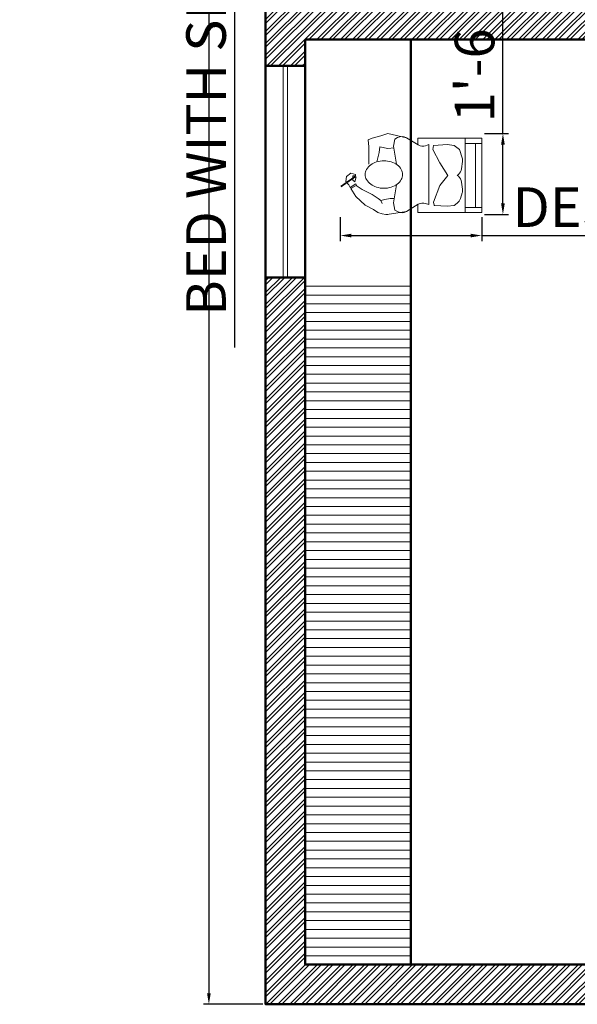
# Model space of a CAD drawing. Units: inches. Extents: x 3590 to 5167, y 65 to 1917.
# Tile 16 of 100: x 3590 to 3716, y 1326 to 1549. Entities that reach past the tile are written whole.
import ezdxf

# ---------------------------------------------------------------- set-up
doc = ezdxf.new("R2010")
doc.units = ezdxf.units.IN
for name, color, linetype, lineweight in [('A-ANNO-DIMS', 2, 'Continuous', 18), ('A-FURN', 21, 'Continuous', 18), ('A-GLAZ', 4, 'Continuous', 18), ('A-WALL', 7, 'Continuous', 50), ('A-WALL-PATT', 251, 'Continuous', 13)]:
    doc.layers.add(name, color=color, linetype=linetype, lineweight=lineweight)
doc.styles.get("Standard").update_dxf_attribs({"font": 'arial.ttf'})
doc.dimstyles.new('ISO-25', dxfattribs={"dimtxt": 9, "dimasz": 2.5, "dimexe": 1.25, "dimexo": 0.625, "dimtad": 1, "dimdec": 1, "dimlunit": 3, "dimtxsty": 'Standard', "dimcen": 2.5, "dimadec": 0, "dimazin": 0, "dimtfac": 1, "dimtdec": 1, "dimtmove": 0, "dimatfit": 3, "dimfxl": 1, "dimarcsym": 0})

# ---------------------------------------------------------------- blocks, each defined once
blk = doc.blocks.new('*D6')
at = {"layer": 'A-ANNO-DIMS', "color": 0, "lineweight": -2, "transparency": 16777216}
for p, q in [((3644.89, 1806), (3631.39, 1806)), ((3632.64, 1803.5), (3632.64, 1328.5)), ((3644.89, 1326), (3631.39, 1326))]:
    blk.add_line(p, q, dxfattribs=at)
at = {"layer": 'A-ANNO-DIMS', "color": 0, "transparency": 16777216}
for points in [[(3632.22, 1803.5), (3633.06, 1803.5), (3632.64, 1806)], [(3632.22, 1328.5), (3633.06, 1328.5), (3632.64, 1326)]]:
    blk.add_solid(points, dxfattribs=at)
at = {"layer": 'Defpoints', "color": 0, "transparency": 16777216}
for p in [(3645.51, 1806), (3632.64, 1326), (3645.51, 1326)]:
    blk.add_point(p, dxfattribs=at)
at = {"layer": 'A-ANNO-DIMS', "color": 0, "transparency": 16777216, "insert": (3627.42, 1566), "char_height": 9, "attachment_point": 5, "rotation": 90}
blk.add_mtext("40'", dxfattribs=at)
blk = doc.blocks.new('DESK-CHAIR')
for p, q in [((3674.9, 1522.4), (3674.54, 1520.79)), ((3675.51, 1522.74), (3674.9, 1522.4)), ((3680.2, 1521.08), (3677.49, 1522.71)), ((3694.59, 1522.58), (3680.09, 1522.58)), ((3680.09, 1522.58), (3680.09, 1521.15)), ((3694.59, 1505.74), (3694.59, 1522.58)), ((3674.54, 1520.79), (3675.25, 1516.67)), ((3682.6, 1521.15), (3681.85, 1520.9)), ((3682.6, 1521.15), (3682.6, 1507.53)), ((3682.6, 1507.53), (3682.6, 1521.15)), ((3683.49, 1520.07), (3683.66, 1520.91)), ((3685.1, 1517.02), (3683.49, 1520.07)), ((3683.73, 1520.97), (3686.72, 1521.15)), ((3686.72, 1521.15), (3688.33, 1520.97)), ((3688.33, 1520.97), (3689.58, 1520.07)), ((3689.58, 1520.07), (3690.17, 1518.15)), ((3686.89, 1514.16), (3685.1, 1517.02)), ((3690.24, 1517.32), (3690.04, 1515.67)), ((3685.1, 1511.83), (3686.89, 1514.16)), ((3689.31, 1514.37), (3689.04, 1514.16)), ((3689.31, 1513.95), (3689.04, 1514.16)), ((3664.74, 1511.43), (3666.04, 1512.26)), ((3665.07, 1511.29), (3664.74, 1511.43)), ((3664.84, 1511.19), (3666.07, 1511.86)), ((3666.04, 1509.36), (3664.84, 1511.19)), ((3666.04, 1512.26), (3666.24, 1511.79)), ((3666.07, 1511.86), (3667.43, 1510.93)), ((3667.43, 1510.93), (3669.7, 1509.83)), ((3674.54, 1507.89), (3675.25, 1512.01)), ((3683.67, 1508.07), (3685.1, 1511.83)), ((3690.24, 1511), (3690.04, 1512.64)), ((3668.13, 1507.37), (3666.04, 1509.36)), ((3669.7, 1509.83), (3671.06, 1508.9)), ((3671.06, 1508.9), (3671.66, 1508.47)), ((3689.78, 1508.89), (3690.17, 1510.17)), ((3670.06, 1506.4), (3668.13, 1507.37)), ((3671.66, 1508.47), (3671.96, 1507.77)), ((3674.9, 1506.27), (3674.54, 1507.89)), ((3680.2, 1507.6), (3677.49, 1505.97)), ((3680.09, 1507.53), (3680.09, 1505.74)), ((3682.6, 1507.53), (3681.85, 1507.78)), ((3683.8, 1507.4), (3683.67, 1508.07)), ((3683.88, 1507.34), (3686.72, 1507.17)), ((3686.72, 1507.17), (3688.33, 1507.35)), ((3688.33, 1507.35), (3689.03, 1507.86)), ((3677.49, 1505.97), (3673.14, 1505.31)), ((3675.51, 1505.94), (3674.9, 1506.27)), ((3680.09, 1505.74), (3694.59, 1505.74))]:
    blk.add_line(p, q)
for points in [[(3677.49, 1522.71), (3673.28, 1523.65), (3671.67, 1523.12), (3669.7, 1522.58), (3668.81, 1522.22), (3668.99, 1520.61), (3668.99, 1519), (3668.99, 1516.67)], [(3664.74, 1511.43), (3664.42, 1512.05), (3663.77, 1512.78), (3663.87, 1513.9), (3664.88, 1514.67), (3665.92, 1514.37), (3665.9, 1514.02), (3665.32, 1514.02), (3665.3, 1513.1), (3665.82, 1512.66), (3666.07, 1513.84)], [(3671.66, 1508.47), (3672.6, 1508.69), (3673.82, 1508.93), (3674.7, 1508.93)], [(3670.06, 1506.4), (3671.04, 1505.75), (3672.02, 1505.46), (3672.8, 1505.31), (3673.24, 1505.31)]]:
    blk.add_lwpolyline(points)
at = {"const_width": 0.39}
blk.add_lwpolyline([(3666.01, 1513.98), (3662.61, 1511.61)], dxfattribs=at)
for centre, radius, start, end in [((3676.47, 1521), 1.98, 59.0235, 119.0669), ((3681.22, 1522.78), 1.98, 239.0235, 288.4436), ((3683.74, 1520.89), 0.0779, 93.3682, 168.6956), ((3683.74, 1520.89), 0.0779, 93.3682, 168.6956), ((3688.27, 1517.56), 1.98, 352.8785, 17.0946), ((3688.07, 1515.92), 1.98, 308.6739, 352.8785), ((3688.07, 1512.4), 1.98, 7.1215, 51.3261), ((3688.27, 1510.75), 1.98, 342.9054, 7.1215), ((3687.88, 1509.47), 1.98, 305.5514, 342.9054), ((3681.22, 1505.89), 1.98, 71.5564, 120.9765), ((3683.88, 1507.42), 0.0779, 191.3044, 266.6318), ((3676.47, 1507.67), 1.98, 240.9331, 300.9765)]:
    blk.add_arc(centre, radius, start, end)
blk = doc.blocks.new('*D286')
at = {"layer": 'A-ANNO-DIMS', "color": 0, "lineweight": -2, "transparency": 16777216}
for p, q in [((3653.89, 1797), (3637.19, 1797)), ((3638.44, 1794.5), (3638.44, 1692.33)), ((3653.89, 1689.83), (3637.19, 1689.83)), ((3638.44, 1689.83), (3638.44, 1475.12))]:
    blk.add_line(p, q, dxfattribs=at)
at = {"layer": 'A-ANNO-DIMS', "color": 0, "transparency": 16777216}
for points in [[(3638.02, 1794.5), (3638.85, 1794.5), (3638.44, 1797)], [(3638.02, 1692.33), (3638.85, 1692.33), (3638.44, 1689.83)]]:
    blk.add_solid(points, dxfattribs=at)
at = {"layer": 'Defpoints', "color": 0, "transparency": 16777216}
for p in [(3654.51, 1797), (3638.44, 1689.83), (3654.51, 1689.83)]:
    blk.add_point(p, dxfattribs=at)
at = {"layer": 'A-ANNO-DIMS', "color": 0, "transparency": 16777216, "insert": (3633.16, 1581.22), "char_height": 9, "attachment_point": 5, "rotation": 90}
blk.add_mtext('BED WITH SIDE TABLES 8\'-11" TYP.', dxfattribs=at)
blk = doc.blocks.new('*D302')
at = {"layer": 'A-ANNO-DIMS', "color": 0, "lineweight": -2, "transparency": 16777216}
for p, q in [((3662.49, 1504.69), (3662.49, 1499.25)), ((3694.59, 1504.69), (3694.59, 1499.25)), ((3664.99, 1500.5), (3692.09, 1500.5)), ((3694.59, 1500.5), (3833.1, 1500.5))]:
    blk.add_line(p, q, dxfattribs=at)
at = {"layer": 'A-ANNO-DIMS', "color": 0, "transparency": 16777216}
for points in [[(3664.99, 1500.91), (3664.99, 1500.08), (3662.49, 1500.5)], [(3692.09, 1500.91), (3692.09, 1500.08), (3694.59, 1500.5)]]:
    blk.add_solid(points, dxfattribs=at)
at = {"layer": 'Defpoints', "color": 0, "transparency": 16777216}
for p in [(3662.49, 1505.31), (3694.59, 1505.31), (3694.59, 1500.5)]:
    blk.add_point(p, dxfattribs=at)
at = {"layer": 'A-ANNO-DIMS', "color": 0, "transparency": 16777216, "insert": (3765.1, 1505.78), "char_height": 9, "attachment_point": 5}
blk.add_mtext('DESK CHAIR 2\'-8" TYP.', dxfattribs=at)
blk = doc.blocks.new('*D303')
at = {"layer": 'A-ANNO-DIMS', "color": 0, "lineweight": -2, "transparency": 16777216}
for p, q in [((3699.41, 1523.65), (3699.41, 1602.39)), ((3695.22, 1523.65), (3700.66, 1523.65)), ((3699.41, 1507.81), (3699.41, 1521.15)), ((3695.22, 1505.31), (3700.66, 1505.31))]:
    blk.add_line(p, q, dxfattribs=at)
at = {"layer": 'A-ANNO-DIMS', "color": 0, "transparency": 16777216}
for points in [[(3698.99, 1521.15), (3699.83, 1521.15), (3699.41, 1523.65)], [(3698.99, 1507.81), (3699.83, 1507.81), (3699.41, 1505.31)]]:
    blk.add_solid(points, dxfattribs=at)
at = {"layer": 'Defpoints', "color": 0, "transparency": 16777216}
for p in [(3694.59, 1523.65), (3699.41, 1523.65), (3694.59, 1505.31)]:
    blk.add_point(p, dxfattribs=at)
at = {"layer": 'A-ANNO-DIMS', "color": 0, "transparency": 16777216, "insert": (3694.13, 1564.27), "char_height": 9, "attachment_point": 5, "rotation": 90}
blk.add_mtext('1\'-6 1/2" TYP.', dxfattribs=at)

msp = doc.modelspace()

# ---------------------------------------------------------------- hatches: boundary and pattern name
at = {"layer": 'A-WALL-PATT', "transparency": 33554687}
h = msp.add_hatch(dxfattribs=at)
h.set_pattern_fill('ANSI32', color=256, scale=0.2)
h.paths.add_polyline_path([(3768.51, 1806), (3645.51, 1806), (3645.51, 1785), (3654.51, 1785), (3654.51, 1797), (3671.16, 1797), (3768.51, 1797)])
h.paths.add_polyline_path([(3909.51, 1806), (3816.51, 1806), (3816.51, 1797), (3864.51, 1797), (3864.51, 1791), (3873.51, 1791), (3873.51, 1797), (3909.51, 1797)])
h.paths.add_polyline_path([(4053.51, 1806), (3969.51, 1806), (3969.51, 1797), (4053.51, 1797)])
h.paths.add_polyline_path([(4215.51, 1806), (4113.51, 1806), (4113.51, 1797), (4206.51, 1797), (4206.51, 1791), (4215.51, 1791)])
h.paths.add_polyline_path([(3654.51, 1737), (3645.51, 1737), (3645.51, 1620), (3654.51, 1620), (3654.51, 1650), (3741.51, 1650), (3741.51, 1656), (3654.51, 1656)], flags=17)
h.paths.add_polyline_path([(3873.51, 1755), (3864.51, 1755), (3864.51, 1656), (3771.51, 1656), (3771.51, 1650), (3774.51, 1650), (3774.51, 1554), (3654.51, 1554), (3654.51, 1584), (3645.51, 1584), (3645.51, 1539), (3654.51, 1539), (3654.51, 1545), (3864.51, 1545), (3864.51, 1539), (3873.51, 1539), (3873.51, 1584), (3864.51, 1584), (3864.51, 1554), (3780.51, 1554), (3780.51, 1650), (3864.51, 1650), (3864.51, 1620), (3873.51, 1620)])
h.paths.add_polyline_path([(3654.51, 1491), (3645.51, 1491), (3645.51, 1326), (3810.51, 1326), (3810.51, 1335), (3809.96, 1335), (3654.51, 1335)])
h.paths.add_polyline_path([(3915.51, 1335), (3873.51, 1335), (3873.51, 1352.87), (3873.51, 1422), (3876.51, 1422), (3876.51, 1431), (3864.51, 1431), (3864.51, 1335), (3858.51, 1335), (3858.51, 1326), (3915.51, 1326)])
h.paths.add_polyline_path([(4028.01, 1335), (4002.51, 1335), (4002.51, 1503), (3981.51, 1503), (3981.51, 1494), (3993.51, 1494), (3993.51, 1431), (3921.51, 1431), (3921.51, 1494), (3933.51, 1494), (3933.51, 1503), (3864.51, 1503), (3864.51, 1494), (3912.51, 1494), (3912.51, 1431), (3906.51, 1431), (3906.51, 1422), (3993.51, 1422), (3993.51, 1335), (3951.51, 1335), (3951.51, 1326), (4028.01, 1326)])
h.paths.add_polyline_path([(4203.51, 1335), (4158.51, 1335), (4158.51, 1527), (4194.51, 1527), (4194.51, 1536), (4149.51, 1536), (4149.51, 1335), (4124.01, 1335), (4124.01, 1326), (4203.51, 1326)])
h.paths.add_polyline_path([(4305.51, 1566), (4296.51, 1566), (4296.51, 1536), (4278.64, 1536), (4260.51, 1536), (4260.51, 1527), (4296.51, 1527), (4296.51, 1521), (4305.51, 1521)])
h.paths.add_polyline_path([(4305.51, 1473), (4296.51, 1473), (4296.51, 1335), (4251.51, 1335), (4251.51, 1326), (4305.51, 1326)])
h.paths.add_polyline_path([(4305.51, 1677), (4215.51, 1677), (4215.51, 1743), (4206.51, 1743), (4206.51, 1677), (4149.51, 1677), (4149.51, 1668), (4296.51, 1668), (4296.51, 1638), (4305.51, 1638)])

# ---------------------------------------------------------------- linework, layer by layer
at = {"layer": 'A-FURN'}
for p, q in [((3690.83, 1505.74), (3690.83, 1522.58)), ((3690.83, 1521.43), (3694.59, 1521.43)), ((3693.16, 1506.84), (3693.16, 1521.43)), ((3690.83, 1506.84), (3694.59, 1506.84)), ((3678.51, 1489), (3654.51, 1489)), ((3678.51, 1487), (3654.51, 1487)), ((3678.51, 1485), (3654.51, 1485)), ((3678.51, 1483), (3654.51, 1483)), ((3678.51, 1481), (3654.51, 1481)), ((3678.51, 1479), (3654.51, 1479)), ((3678.51, 1477), (3654.51, 1477)), ((3678.51, 1475), (3654.51, 1475)), ((3678.51, 1473), (3654.51, 1473)), ((3678.51, 1471), (3654.51, 1471)), ((3678.51, 1469), (3654.51, 1469)), ((3678.51, 1467), (3654.51, 1467)), ((3678.51, 1465), (3654.51, 1465)), ((3678.51, 1463), (3654.51, 1463)), ((3678.51, 1461), (3654.51, 1461)), ((3678.51, 1459), (3654.51, 1459)), ((3678.51, 1457), (3654.51, 1457)), ((3678.51, 1455), (3654.51, 1455)), ((3678.51, 1453), (3654.51, 1453)), ((3678.51, 1451), (3654.51, 1451)), ((3678.51, 1449), (3654.51, 1449)), ((3678.51, 1447), (3654.51, 1447)), ((3678.51, 1445), (3654.51, 1445)), ((3678.51, 1443), (3654.51, 1443)), ((3678.51, 1441), (3654.51, 1441)), ((3678.51, 1439), (3654.51, 1439)), ((3678.51, 1437), (3654.51, 1437)), ((3678.51, 1435), (3654.51, 1435)), ((3678.51, 1433), (3654.51, 1433)), ((3678.51, 1431), (3654.51, 1431)), ((3678.51, 1429), (3654.51, 1429)), ((3678.51, 1427), (3654.51, 1427)), ((3678.51, 1425), (3654.51, 1425)), ((3678.51, 1423), (3654.51, 1423)), ((3678.51, 1421), (3654.51, 1421)), ((3678.51, 1419), (3654.51, 1419)), ((3678.51, 1417), (3654.51, 1417)), ((3678.51, 1415), (3654.51, 1415)), ((3678.51, 1413), (3654.51, 1413)), ((3678.51, 1411), (3654.51, 1411)), ((3678.51, 1409), (3654.51, 1409)), ((3678.51, 1407), (3654.51, 1407)), ((3678.51, 1405), (3654.51, 1405)), ((3678.51, 1403), (3654.51, 1403)), ((3678.51, 1401), (3654.51, 1401)), ((3678.51, 1399), (3654.51, 1399)), ((3678.51, 1397), (3654.51, 1397)), ((3678.51, 1395), (3654.51, 1395)), ((3678.51, 1393), (3654.51, 1393)), ((3678.51, 1391), (3654.51, 1391)), ((3678.51, 1389), (3654.51, 1389)), ((3678.51, 1387), (3654.51, 1387)), ((3678.51, 1385), (3654.51, 1385)), ((3678.51, 1383), (3654.51, 1383)), ((3678.51, 1381), (3654.51, 1381)), ((3678.51, 1379), (3654.51, 1379)), ((3678.51, 1377), (3654.51, 1377)), ((3678.51, 1375), (3654.51, 1375)), ((3678.51, 1373), (3654.51, 1373)), ((3678.51, 1371), (3654.51, 1371)), ((3678.51, 1369), (3654.51, 1369)), ((3678.51, 1367), (3654.51, 1367)), ((3678.51, 1365), (3654.51, 1365)), ((3678.51, 1363), (3654.51, 1363)), ((3678.51, 1361), (3654.51, 1361)), ((3678.51, 1359), (3654.51, 1359)), ((3678.51, 1357), (3654.51, 1357)), ((3678.51, 1355), (3654.51, 1355)), ((3678.51, 1353), (3654.51, 1353)), ((3678.51, 1351), (3654.51, 1351)), ((3678.51, 1349), (3654.51, 1349)), ((3678.51, 1347), (3654.51, 1347)), ((3678.51, 1345), (3654.51, 1345)), ((3678.51, 1343), (3654.51, 1343)), ((3678.51, 1343), (3654.51, 1343)), ((3678.51, 1341), (3654.51, 1341)), ((3678.51, 1339), (3654.51, 1339)), ((3678.51, 1337), (3654.51, 1337))]:
    msp.add_line(p, q, dxfattribs=at)
msp.add_lwpolyline([(3670.78, 1517.2), (3671.31, 1519.35), (3671.49, 1520.61), (3673.28, 1520.25), (3674.72, 1520.43)], dxfattribs=at)
msp.add_lwpolyline([(3672.39, 1511.23, 0.07405), (3674.07, 1511.48, 0.084801), (3675.39, 1512.14, 0.106336), (3676.34, 1513.21, 0.128955), (3676.64, 1514.35, 0.128955), (3676.34, 1515.49, 0.106336), (3675.39, 1516.56, 0.084801), (3674.07, 1517.22, 0.07405), (3672.39, 1517.47, 0.07405), (3670.71, 1517.22, 0.084801), (3669.39, 1516.56, 0.106336), (3668.44, 1515.49, 0.128955), (3668.14, 1514.35, 0.128955), (3668.44, 1513.21, 0.106336), (3669.39, 1512.14, 0.084801), (3670.71, 1511.48, 0.07405)], format="xyb", close=True, dxfattribs=at)
at = {"layer": 'A-GLAZ'}
for p, q in [((3649.51, 1491), (3649.51, 1539)), ((3650.51, 1491), (3650.51, 1539))]:
    msp.add_line(p, q, dxfattribs=at)
at = {"layer": 'A-WALL'}
for p, q in [((3654.51, 1335), (3654.51, 1545)), ((3864.51, 1545), (3654.51, 1545)), ((3678.51, 1335), (3678.51, 1545)), ((3654.51, 1539), (3645.51, 1539)), ((3654.51, 1491), (3645.51, 1491)), ((3864.51, 1335), (3654.51, 1335))]:
    msp.add_line(p, q, dxfattribs=at)
msp.add_lwpolyline([(4305.51, 1677), (4305.51, 1326), (3645.51, 1326), (3645.51, 1806), (4215.51, 1806)], dxfattribs=at)

# ---------------------------------------------------------------- block references
at = {"layer": 'A-FURN'}
msp.add_blockref('DESK-CHAIR', (0, 0), dxfattribs=at)

# ---------------------------------------------------------------- dimensions: what is measured, and where the dimension line sits
at = {"layer": 'A-ANNO-DIMS'}
dim = msp.add_linear_dim(base=(3632.64, 1326), p1=(3645.51, 1806), p2=(3645.51, 1326), angle=90, dimstyle='ISO-25', override={"dimclrd": 0, "dimclre": 0, "dimclrt": 0}, dxfattribs=at)
dim.commit()
dim.dimension.update_dxf_attribs({"geometry": '*D6', "text_midpoint": (3627.42, 1566)})
for base, p1, p2, angle, text, picture, middle in [((3638.44, 1689.83), (3654.51, 1797), (3654.51, 1689.83), 270, 'BED WITH SIDE TABLES <> TYP.', '*D286', (3633.16, 1581.22)), ((3699.41, 1523.65), (3694.59, 1505.31), (3694.59, 1523.65), 90, '<> TYP.', '*D303', (3694.13, 1564.27))]:
    dim = msp.add_linear_dim(base=base, p1=p1, p2=p2, angle=angle, text=text, dimstyle='ISO-25', override={"dimdec": 1, "dimlfac": 1, "dimrnd": 0, "dimzin": 1, "dimdsep": 46, "dimlunit": 4, "dimfrac": 2}, dxfattribs=at)
    dim.commit()
    dim.dimension.update_dxf_attribs({"geometry": picture, "text_midpoint": middle})
dim = msp.add_linear_dim(base=(3694.59, 1500.5), p1=(3662.49, 1505.31), p2=(3694.59, 1505.31), text='DESK CHAIR <> TYP.', dimstyle='ISO-25', override={"dimdec": 1, "dimlfac": 1, "dimrnd": 0, "dimzin": 1, "dimdsep": 46, "dimlunit": 4, "dimfrac": 2}, dxfattribs=at)
dim.commit()
dim.dimension.update_dxf_attribs({"geometry": '*D302', "text_midpoint": (3765.1, 1505.78)})

doc.saveas('drawing.dxf')
